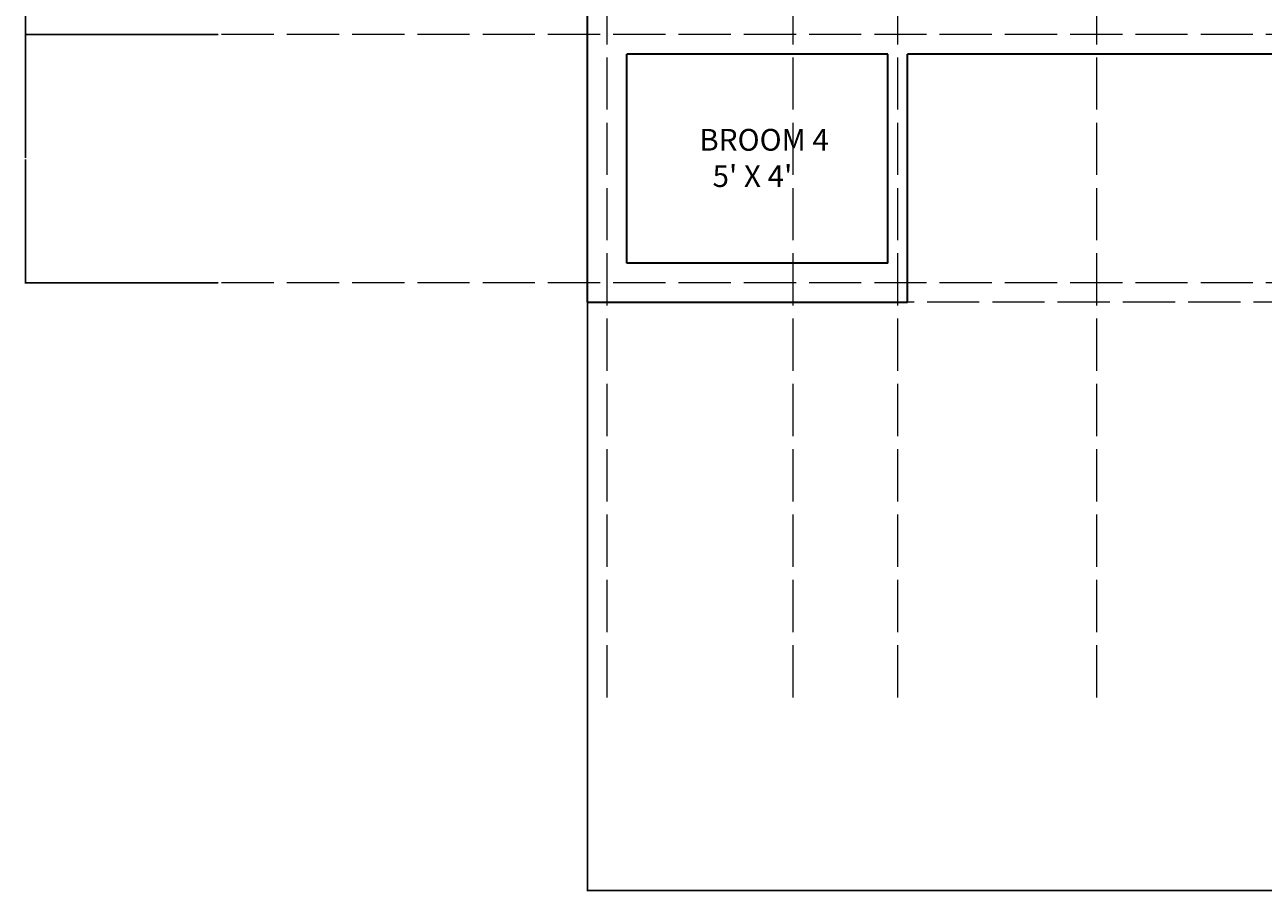
# Model space of a CAD drawing. Units: inches. Extents: x 1159 to 4240, y 1112 to 2085.
# Tile 1 of 13: x 1159 to 1443, y 1112 to 1311. Entities that reach past the tile are written whole.
import ezdxf

# ---------------------------------------------------------------- set-up
doc = ezdxf.new("R2010")
doc.units = ezdxf.units.IN
doc.linetypes.add('ACAD_ISO02W100', pattern=[15, 12, -3])
for name, color, linetype, lineweight in [('A-ANNO-DIMS', 2, 'Continuous', 18), ('A-AREA-IDEN', 30, 'Continuous', 18), ('A-FLOR-EDGE', 1, 'ACAD_ISO02W100', 18), ('A-GRID', 8, 'ACAD_ISO02W100', 13), ('WALL', 7, 'Continuous', 35)]:
    doc.layers.add(name, color=color, linetype=linetype, lineweight=lineweight)
doc.styles.get("Standard").update_dxf_attribs({"font": 'arial.ttf'})
doc.dimstyles.get("Standard").update_dxf_attribs({"dimtxt": 0.18, "dimasz": 0.18, "dimexe": 0.18, "dimexo": 0.0625, "dimgap": 0.09, "dimtad": 0, "dimtih": 1, "dimtoh": 1, "dimdec": 4, "dimzin": 0, "dimdsep": 46, "dimtxsty": 'Standard', "dimcen": 0.09, "dimadec": 0, "dimazin": 0, "dimtfac": 1, "dimtdec": 4, "dimtofl": 0, "dimtmove": 0, "dimatfit": 3, "dimfxl": 1, "dimtolj": 1, "dimtzin": 0, "dimarcsym": 0})

# ---------------------------------------------------------------- blocks, each defined once
blk = doc.blocks.new('HOUSE-35x60-WALL-LAYOUT')
for p, q in [((0, 0), (0, 720)), ((9, 9), (9, 57)), ((69, 57), (9, 57)), ((69, 9), (69, 57)), ((162, 57), (73.5, 57)), ((73.5, 0), (73.5, 57)), ((69, 9), (9, 9)), ((0, 0), (73.5, 0))]:
    blk.add_line(p, q)
blk = doc.blocks.new('HOUSE-35x60-SETTING-OUT-GRID')
for p, q in [((89.32, 0), (89.32, 883.25)), ((132.07, 0), (132.07, 883.25)), ((156.07, 0), (156.07, 883.25)), ((201.82, 0), (201.82, 883.25)), ((582.7, 152.25), (0, 152.25)), ((582.7, 95.25), (0, 95.25))]:
    blk.add_line(p, q)
blk = doc.blocks.new('*D22')
at = {"layer": 'A-ANNO-DIMS', "color": 0, "lineweight": -2, "transparency": 16777216}
for p, q in [((1288.13, 1247.64), (1288.13, 1112.42)), ((1708.13, 1247.64), (1708.13, 1112.42)), ((1288.31, 1112.6), (1497.83, 1112.6)), ((1707.95, 1112.6), (1498.42, 1112.6))]:
    blk.add_line(p, q, dxfattribs=at)
at = {"layer": 'A-ANNO-DIMS', "color": 0, "lineweight": 100, "transparency": 16777216}
for points in [[(1288.31, 1112.63), (1288.31, 1112.57), (1288.13, 1112.6)], [(1707.95, 1112.63), (1707.95, 1112.57), (1708.13, 1112.6)]]:
    blk.add_solid(points, dxfattribs=at)
at = {"layer": 'Defpoints', "color": 0, "lineweight": 100, "transparency": 16777216}
for p in [(1288.13, 1247.7), (1708.13, 1247.7), (1708.13, 1112.6)]:
    blk.add_point(p, dxfattribs=at)
at = {"layer": 'A-ANNO-DIMS', "color": 0, "transparency": 16777216, "insert": (1498.13, 1112.6), "char_height": 0.18, "attachment_point": 5}
blk.add_mtext('\\A1;420', dxfattribs=at)
blk = doc.blocks.new('*D37')
at = {"layer": 'A-ANNO-DIMS', "color": 0, "lineweight": -2, "transparency": 16777216}
for p, q in [((1203.25, 1309.2), (1158.78, 1309.2)), ((1158.96, 1309.02), (1158.96, 1280.88)), ((1158.96, 1252.38), (1158.96, 1280.52)), ((1203.25, 1252.2), (1158.78, 1252.2))]:
    blk.add_line(p, q, dxfattribs=at)
at = {"layer": 'A-ANNO-DIMS', "color": 0, "lineweight": 100, "transparency": 16777216}
for points in [[(1158.93, 1309.02), (1158.99, 1309.02), (1158.96, 1309.2)], [(1158.93, 1252.38), (1158.99, 1252.38), (1158.96, 1252.2)]]:
    blk.add_solid(points, dxfattribs=at)
at = {"layer": 'Defpoints', "color": 0, "lineweight": 100, "transparency": 16777216}
for p in [(1158.96, 1309.2), (1203.31, 1309.2), (1203.31, 1252.2)]:
    blk.add_point(p, dxfattribs=at)
at = {"layer": 'A-ANNO-DIMS', "color": 0, "transparency": 16777216, "insert": (1158.96, 1280.7), "char_height": 0.18, "attachment_point": 5}
blk.add_mtext('\\A1;57', dxfattribs=at)
blk = doc.blocks.new('*D38')
at = {"layer": 'A-ANNO-DIMS', "color": 0, "lineweight": -2, "transparency": 16777216}
for p, q in [((1203.25, 1366.2), (1158.78, 1366.2)), ((1158.96, 1366.02), (1158.96, 1337.88)), ((1158.96, 1309.38), (1158.96, 1337.52)), ((1203.25, 1309.2), (1158.78, 1309.2))]:
    blk.add_line(p, q, dxfattribs=at)
at = {"layer": 'A-ANNO-DIMS', "color": 0, "lineweight": 100, "transparency": 16777216}
for points in [[(1158.93, 1366.02), (1158.99, 1366.02), (1158.96, 1366.2)], [(1158.93, 1309.38), (1158.99, 1309.38), (1158.96, 1309.2)]]:
    blk.add_solid(points, dxfattribs=at)
at = {"layer": 'Defpoints', "color": 0, "lineweight": 100, "transparency": 16777216}
for p in [(1158.96, 1366.2), (1203.31, 1366.2), (1203.31, 1309.2)]:
    blk.add_point(p, dxfattribs=at)
at = {"layer": 'A-ANNO-DIMS', "color": 0, "transparency": 16777216, "insert": (1158.96, 1337.7), "char_height": 0.18, "attachment_point": 5}
blk.add_mtext('\\A1;57', dxfattribs=at)

msp = doc.modelspace()

# ---------------------------------------------------------------- linework, layer by layer
at = {"layer": 'A-FLOR-EDGE'}
msp.add_line((1708.125, 1247.702), (1361.625, 1247.702), dxfattribs=at)

# ---------------------------------------------------------------- block references
at = {"layer": 'A-GRID'}
msp.add_blockref('HOUSE-35x60-SETTING-OUT-GRID', (1203.31, 1156.954), dxfattribs=at)
at = {"layer": 'WALL'}
msp.add_blockref('HOUSE-35x60-WALL-LAYOUT', (1288.126, 1247.702), dxfattribs=at)

# ---------------------------------------------------------------- texts
at = {"layer": 'A-AREA-IDEN', "insert": (1313.772, 1287.528), "char_height": 5, "attachment_point": 1}
msp.add_mtext_dynamic_manual_height_columns("\\A1;BROOM 4 \\P  5' X 4'", width=140.18614, gutter_width=12.5, heights=[0], dxfattribs=at)

# ---------------------------------------------------------------- dimensions: what is measured, and where the dimension line sits
at = {"layer": 'A-ANNO-DIMS'}
for base, p1, p2, picture, middle in [((1158.96, 1366.202), (1203.31, 1309.202), (1203.31, 1366.202), '*D38', (1158.96, 1337.702)), ((1158.96, 1309.202), (1203.31, 1252.202), (1203.31, 1309.202), '*D37', (1158.96, 1280.702))]:
    dim = msp.add_linear_dim(base=base, p1=p1, p2=p2, angle=90, dimstyle='Standard', override={"dimdec": 0, "dimlfac": 1, "dimrnd": 0, "dimzin": 0, "dimdsep": 46, "dimlunit": 2}, dxfattribs=at)
    dim.commit()
    dim.dimension.update_dxf_attribs({"geometry": picture, "text_midpoint": middle})
dim = msp.add_linear_dim(base=(1708.125, 1112.604), p1=(1288.125, 1247.702), p2=(1708.125, 1247.702), dimstyle='Standard', override={"dimdec": 0, "dimlfac": 1, "dimrnd": 0, "dimzin": 0, "dimdsep": 46, "dimlunit": 2}, dxfattribs=at)
dim.commit()
dim.dimension.update_dxf_attribs({"geometry": '*D22', "text_midpoint": (1498.125, 1112.604)})

doc.saveas('drawing.dxf')
